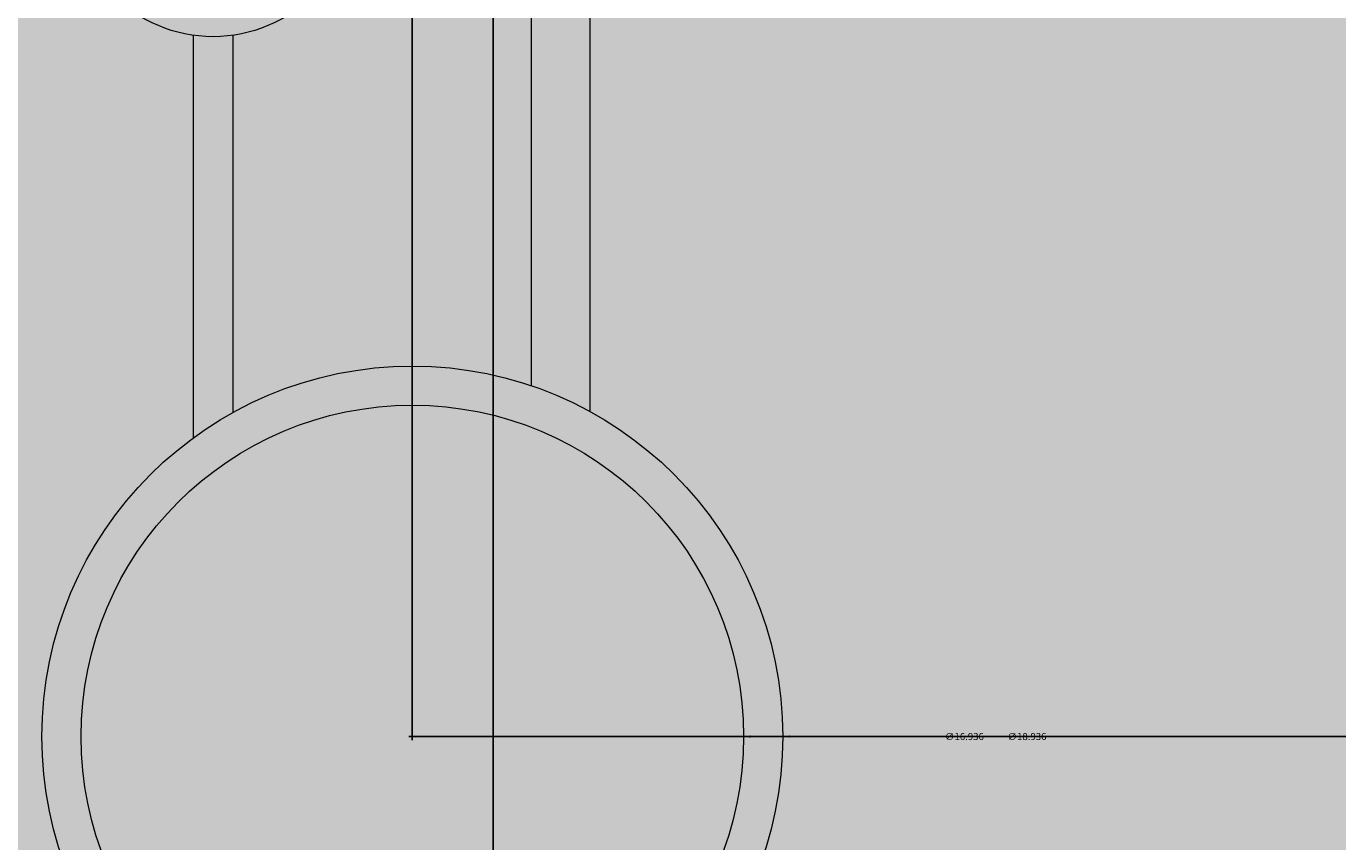
# Model space of a CAD drawing. Units: inches. Extents: x 4508 to 4723, y 847 to 1020.
# Tile 27 of 32: x 4657 to 4691, y 933 to 954. Entities that reach past the tile are written whole.
import ezdxf

# ---------------------------------------------------------------- set-up
doc = ezdxf.new("R2010")
doc.units = ezdxf.units.IN
for name, color, linetype, lineweight in [('A-ANNO-DIMS', 2, 'Continuous', 18), ('A-WALL-DECO', 6, 'Continuous', 18), ('A-WALL-PATT', 254, 'Continuous', 13)]:
    doc.layers.add(name, color=color, linetype=linetype, lineweight=lineweight)
doc.styles.get("Standard").update_dxf_attribs({"font": 'arial.ttf'})
doc.dimstyles.get("Standard").update_dxf_attribs({"dimtxt": 0.18, "dimasz": 0.18, "dimexe": 0.18, "dimexo": 0.0625, "dimgap": 0.09, "dimtad": 0, "dimtih": 1, "dimtoh": 1, "dimdec": 4, "dimzin": 0, "dimdsep": 46, "dimtxsty": 'Standard', "dimcen": 0.09, "dimadec": 0, "dimazin": 0, "dimtfac": 1, "dimtdec": 4, "dimtofl": 0, "dimtmove": 0, "dimatfit": 3, "dimfxl": 1, "dimtolj": 1, "dimtzin": 0, "dimarcsym": 0})

# ---------------------------------------------------------------- blocks, each defined once
blk = doc.blocks.new('*D8')
at = {"layer": 'A-ANNO-DIMS', "color": 0, "lineweight": -2, "transparency": 16777216}
for p, q in [((4662.171, 957.665), (4662.171, 1002.877)), ((4662.351, 1002.697), (4664.34, 1002.697)), ((4667.082, 1002.697), (4665.092, 1002.697)), ((4667.262, 936.184), (4667.262, 1002.877))]:
    blk.add_line(p, q, dxfattribs=at)
at = {"layer": 'A-ANNO-DIMS', "color": 0, "lineweight": 9, "transparency": 16777216}
for points in [[(4662.351, 1002.727), (4662.351, 1002.667), (4662.171, 1002.697)], [(4667.082, 1002.727), (4667.082, 1002.667), (4667.262, 1002.697)]]:
    blk.add_solid(points, dxfattribs=at)
at = {"layer": 'Defpoints', "color": 0, "lineweight": 9, "transparency": 16777216}
for p in [(4667.262, 1002.697), (4662.171, 957.602), (4667.262, 936.122)]:
    blk.add_point(p, dxfattribs=at)
at = {"layer": 'A-ANNO-DIMS', "color": 0, "transparency": 16777216, "insert": (4664.716, 1002.697), "char_height": 0.18, "attachment_point": 5}
blk.add_mtext('\\A1;5.091', dxfattribs=at)
blk = doc.blocks.new('*D9')
at = {"layer": 'A-ANNO-DIMS', "color": 0, "lineweight": -2, "transparency": 16777216}
for p, q in [((4667.262, 936.184), (4667.262, 1002.877)), ((4667.442, 1002.697), (4668.461, 1002.697)), ((4670.126, 1002.697), (4669.107, 1002.697)), ((4670.306, 994.809), (4670.306, 1002.877))]:
    blk.add_line(p, q, dxfattribs=at)
at = {"layer": 'A-ANNO-DIMS', "color": 0, "lineweight": 9, "transparency": 16777216}
for points in [[(4667.442, 1002.727), (4667.442, 1002.667), (4667.262, 1002.697)], [(4670.126, 1002.727), (4670.126, 1002.667), (4670.306, 1002.697)]]:
    blk.add_solid(points, dxfattribs=at)
at = {"layer": 'Defpoints', "color": 0, "lineweight": 9, "transparency": 16777216}
for p in [(4670.306, 1002.697), (4670.306, 994.747), (4667.262, 936.122)]:
    blk.add_point(p, dxfattribs=at)
at = {"layer": 'A-ANNO-DIMS', "color": 0, "transparency": 16777216, "insert": (4668.784, 1002.697), "char_height": 0.18, "attachment_point": 5}
blk.add_mtext('\\A1;3.04', dxfattribs=at)
blk = doc.blocks.new('*D13')
at = {"layer": 'A-ANNO-DIMS', "color": 0, "lineweight": -2, "transparency": 16777216}
for p, q in [((4669.325, 973.916), (4669.325, 866.617)), ((4689.994, 874.684), (4689.994, 866.617)), ((4669.505, 866.797), (4679.264, 866.797)), ((4689.814, 866.797), (4680.054, 866.797))]:
    blk.add_line(p, q, dxfattribs=at)
at = {"layer": 'A-ANNO-DIMS', "color": 0, "lineweight": 9, "transparency": 16777216}
for points in [[(4669.505, 866.827), (4669.505, 866.767), (4669.325, 866.797)], [(4689.814, 866.827), (4689.814, 866.767), (4689.994, 866.797)]]:
    blk.add_solid(points, dxfattribs=at)
at = {"layer": 'Defpoints', "color": 0, "lineweight": 9, "transparency": 16777216}
for p in [(4669.325, 973.978), (4689.994, 874.747), (4689.994, 866.797)]:
    blk.add_point(p, dxfattribs=at)
at = {"layer": 'A-ANNO-DIMS', "color": 0, "transparency": 16777216, "insert": (4679.659, 866.797), "char_height": 0.18, "attachment_point": 5}
blk.add_mtext('\\A1;20.67', dxfattribs=at)
blk = doc.blocks.new('*D20')
at = {"layer": 'A-ANNO-DIMS', "color": 0, "lineweight": -2, "transparency": 16777216}
for p, q in [((4667.324, 936.122), (4702.124, 936.122)), ((4701.944, 935.942), (4701.944, 925.563)), ((4701.944, 914.821), (4701.944, 925.2)), ((4662.233, 914.641), (4702.124, 914.641))]:
    blk.add_line(p, q, dxfattribs=at)
at = {"layer": 'A-ANNO-DIMS', "color": 0, "lineweight": 9, "transparency": 16777216}
for points in [[(4701.914, 935.942), (4701.974, 935.942), (4701.944, 936.122)], [(4701.914, 914.821), (4701.974, 914.821), (4701.944, 914.641)]]:
    blk.add_solid(points, dxfattribs=at)
at = {"layer": 'Defpoints', "color": 0, "lineweight": 9, "transparency": 16777216}
for p in [(4667.262, 936.122), (4701.944, 936.122), (4662.171, 914.641)]:
    blk.add_point(p, dxfattribs=at)
at = {"layer": 'A-ANNO-DIMS', "color": 0, "transparency": 16777216, "insert": (4701.944, 925.381), "char_height": 0.18, "attachment_point": 5}
blk.add_mtext('\\A1;21.48', dxfattribs=at)
blk = doc.blocks.new('*D21')
at = {"layer": 'A-ANNO-DIMS', "color": 0, "lineweight": -2, "transparency": 16777216}
for p, q in [((4662.233, 957.602), (4702.124, 957.602)), ((4701.944, 957.422), (4701.944, 947.044)), ((4701.944, 936.302), (4701.944, 946.68)), ((4667.324, 936.122), (4702.124, 936.122))]:
    blk.add_line(p, q, dxfattribs=at)
at = {"layer": 'A-ANNO-DIMS', "color": 0, "lineweight": 9, "transparency": 16777216}
for points in [[(4701.914, 957.422), (4701.974, 957.422), (4701.944, 957.602)], [(4701.914, 936.302), (4701.974, 936.302), (4701.944, 936.122)]]:
    blk.add_solid(points, dxfattribs=at)
at = {"layer": 'Defpoints', "color": 0, "lineweight": 9, "transparency": 16777216}
for p in [(4662.171, 957.602), (4701.944, 957.602), (4667.262, 936.122)]:
    blk.add_point(p, dxfattribs=at)
at = {"layer": 'A-ANNO-DIMS', "color": 0, "transparency": 16777216, "insert": (4701.944, 946.862), "char_height": 0.18, "attachment_point": 5}
blk.add_mtext('\\A1;21.48', dxfattribs=at)
blk = doc.blocks.new('*D42')
at = {"layer": 'A-ANNO-DIMS', "color": 0, "lineweight": -2, "transparency": 16777216}
for p, q in [((4667.172, 936.122), (4667.352, 936.122)), ((4667.262, 936.032), (4667.262, 936.212)), ((4682.411, 936.122), (4676.91, 936.122))]:
    blk.add_line(p, q, dxfattribs=at)
at = {"layer": 'A-ANNO-DIMS', "color": 0, "lineweight": 9, "transparency": 16777216}
blk.add_solid([(4676.91, 936.152), (4676.91, 936.092), (4676.73, 936.122)], dxfattribs=at)
at = {"layer": 'Defpoints', "color": 0, "lineweight": 9, "transparency": 16777216}
for p in [(4657.794, 936.121), (4676.73, 936.122)]:
    blk.add_point(p, dxfattribs=at)
at = {"layer": 'A-ANNO-DIMS', "color": 0, "transparency": 16777216, "insert": (4682.972, 936.122), "char_height": 0.18, "attachment_point": 5}
blk.add_mtext('\\A1;∅18.936', dxfattribs=at)
blk = doc.blocks.new('*D43')
at = {"layer": 'A-ANNO-DIMS', "color": 0, "lineweight": -2, "transparency": 16777216}
for p, q in [((4667.172, 936.122), (4667.352, 936.122)), ((4667.262, 936.032), (4667.262, 936.212)), ((4680.811, 936.122), (4675.91, 936.122))]:
    blk.add_line(p, q, dxfattribs=at)
at = {"layer": 'A-ANNO-DIMS', "color": 0, "lineweight": 9, "transparency": 16777216}
blk.add_solid([(4675.91, 936.152), (4675.91, 936.092), (4675.73, 936.122)], dxfattribs=at)
at = {"layer": 'Defpoints', "color": 0, "lineweight": 9, "transparency": 16777216}
for p in [(4658.794, 936.121), (4675.73, 936.122)]:
    blk.add_point(p, dxfattribs=at)
at = {"layer": 'A-ANNO-DIMS', "color": 0, "transparency": 16777216, "insert": (4681.372, 936.122), "char_height": 0.18, "attachment_point": 5}
blk.add_mtext('\\A1;∅16.936', dxfattribs=at)

msp = doc.modelspace()

# ---------------------------------------------------------------- hatches: boundary and pattern name
at = {"layer": 'A-WALL-PATT', "transparency": 33554508}
h = msp.add_hatch(color=256, dxfattribs=at)
h.dxf.hatch_style = 1
h.paths.add_polyline_path([(4661.6706, 954.043, -0.3739004), (4658.5765, 957.6021, -1), (4665.7646, 957.6021, -0.3739004), (4662.6706, 954.043), (4662.6706, 944.4021, -0.2114781), (4670.3062, 945.0869), (4670.3062, 968.0592, -0.4632086), (4663.3246, 973.9783, -0.4632086), (4670.3062, 979.8975), (4670.3062, 994.7469), (4588.9938, 994.7469), (4588.9938, 904.7469), (4657.9938, 904.7469), (4657.9938, 886.7469), (4549.9938, 886.7469), (4549.9938, 878.7469), (4693.9938, 878.7469), (4693.9938, 994.7469), (4671.8062, 994.7469), (4671.8062, 979.4411, -0.2941682), (4675.3246, 973.9783, -0.2941682), (4671.8062, 968.5156), (4671.8062, 944.4278, -0.2741114), (4676.7298, 936.1217, -0.2741114), (4671.8062, 927.8155), (4671.8062, 907.6998, -0.3779645), (4677.0562, 901.7469, -0.3779645), (4671.8062, 895.7939), (4671.8062, 883.7469), (4670.3062, 883.7469), (4670.3062, 895.7939, -0.3779645), (4665.0562, 901.7469, -0.3779645), (4670.3062, 907.6998), (4670.3062, 927.1564, -0.2114781), (4662.6706, 927.8412), (4662.6706, 918.2003, -0.3739004), (4665.7646, 914.6412, -1), (4658.5765, 914.6412, -0.3739004), (4661.6706, 918.2003), (4661.6706, 928.4807, -0.2391825), (4657.7936, 936.1217, -0.2391825), (4661.6706, 943.7626)])
at = {"layer": 'A-WALL-PATT', "transparency": 33554681}
h = msp.add_hatch(color=256, dxfattribs=at)
h.dxf.hatch_style = 1
h.paths.add_polyline_path([(4671.8062, 968.5156, -0.0656104), (4670.3062, 968.0592), (4670.3062, 945.0869, -0.0433429), (4671.8062, 944.4278)])
h.paths.add_polyline_path([(4662.6706, 954.043, -0.0698991), (4661.6706, 954.043), (4661.6706, 943.7626, -0.0313734), (4662.6706, 944.4021)])
h.paths.add_polyline_path([(4665.7646, 957.6021, 1), (4658.5765, 957.6021, 1)])
h.paths.add_polyline_path([(4659.0765, 957.6021, -1), (4665.2646, 957.6021, -1)], flags=16)
h.paths.add_polyline_path([(4675.3246, 973.9783, 1), (4663.3246, 973.9783, 1)])
h.paths.add_polyline_path([(4664.3246, 973.9783, -1), (4674.3246, 973.9783, -1)], flags=16)
h.paths.add_polyline_path([(4671.8062, 994.7469), (4670.3062, 994.7469), (4670.3062, 979.8975, -0.0656104), (4671.8062, 979.4411)])
at = {"layer": 'A-WALL-PATT', "transparency": 33554556}
h = msp.add_hatch(color=256, dxfattribs=at)
h.dxf.hatch_style = 1
h.paths.add_polyline_path([(4676.0562, 901.7469, 1), (4666.0562, 901.7469, 1)])
h.paths.add_polyline_path([(4659.0765, 914.6412, 1), (4665.2646, 914.6412, 1)])
h.paths.add_polyline_path([(4675.7298, 936.1217, 1), (4658.7936, 936.1217, 1)])
h.paths.add_polyline_path([(4659.0765, 957.6021, 1), (4665.2646, 957.6021, 1)])
h.paths.add_polyline_path([(4664.3246, 973.9783, 1), (4674.3246, 973.9783, 1)])
at = {"layer": 'A-WALL-PATT', "transparency": 33554681}
h = msp.add_hatch(color=256, dxfattribs=at)
h.dxf.hatch_style = 1
h.paths.add_polyline_path([(4676.7298, 936.1217, 1), (4657.7936, 936.1217, 1)])
h.paths.add_polyline_path([(4658.7936, 936.1217, -1), (4675.7298, 936.1217, -1)], flags=16)

# ---------------------------------------------------------------- linework, layer by layer
at = {"layer": 'A-WALL-DECO'}
for p, q in [((4671.8062, 944.4278), (4671.8062, 968.5156)), ((4670.3062, 945.0869), (4670.3062, 968.0592))]:
    msp.add_line(p, q, dxfattribs=at)
for points in [[(4661.6706, 943.7626), (4661.6706, 954.043)], [(4662.6706, 954.043), (4662.6706, 944.4021)]]:
    msp.add_lwpolyline(points, dxfattribs=at)
for centre, radius in [((4662.1706, 957.6021), 3.5941), ((4667.2617, 936.1217), 9.4681), ((4667.2617, 936.1217), 8.4681)]:
    msp.add_circle(centre, radius, dxfattribs=at)

# ---------------------------------------------------------------- dimensions: what is measured, and where the dimension line sits
at = {"layer": 'A-ANNO-DIMS'}
for base, p1, p2, override, picture, middle in [((4667.2617, 1002.6969), (4662.1706, 957.6021), (4667.2617, 936.1217), {"dimdec": 3, "dimlfac": 1, "dimrnd": 0, "dimzin": 0, "dimdsep": 46, "dimlunit": 2}, '*D8', (4664.7161, 1002.6969)), ((4670.3062, 1002.6969), (4667.2617, 936.1217), (4670.3062, 994.7469), {"dimdec": 2, "dimlfac": 1, "dimrnd": 0, "dimzin": 0, "dimdsep": 46, "dimlunit": 2}, '*D9', (4668.7839, 1002.6969)), ((4689.9938, 866.7969), (4669.3246, 973.9783), (4689.9938, 874.7469), {"dimdec": 2, "dimlfac": 1, "dimrnd": 0, "dimzin": 0, "dimdsep": 46, "dimlunit": 2}, '*D13', (4679.6592, 866.7969))]:
    dim = msp.add_linear_dim(base=base, p1=p1, p2=p2, dimstyle='Standard', override=override, dxfattribs=at)
    dim.commit()
    dim.dimension.update_dxf_attribs({"geometry": picture, "text_midpoint": middle})
for base, p1, p2, picture, middle in [((4701.9438, 957.6021), (4667.2617, 936.1217), (4662.1706, 957.6021), '*D21', (4701.9438, 946.8619)), ((4701.9438, 936.1217), (4662.1706, 914.6412), (4667.2617, 936.1217), '*D20', (4701.9438, 925.3814))]:
    dim = msp.add_linear_dim(base=base, p1=p1, p2=p2, angle=90, dimstyle='Standard', override={"dimdec": 2, "dimlfac": 1, "dimrnd": 0, "dimzin": 0, "dimdsep": 46, "dimlunit": 2}, dxfattribs=at)
    dim.commit()
    dim.dimension.update_dxf_attribs({"geometry": picture, "text_midpoint": middle})
for p1, p2, picture, middle in [((4657.7936, 936.1213), (4676.7298, 936.122), '*D42', (4682.4106, 936.1222)), ((4658.7936, 936.1213), (4675.7298, 936.122), '*D43', (4680.8106, 936.1222))]:
    dim = msp.add_diameter_dim_2p(p1=p1, p2=p2, dimstyle='Standard', override={"dimdec": 3, "dimlfac": 1, "dimrnd": 0, "dimzin": 0, "dimdsep": 46, "dimlunit": 2}, dxfattribs=at)
    dim.commit()
    dim.dimension.update_dxf_attribs({"geometry": picture, "text_midpoint": middle, "dimtype": 163})

doc.saveas('drawing.dxf')
